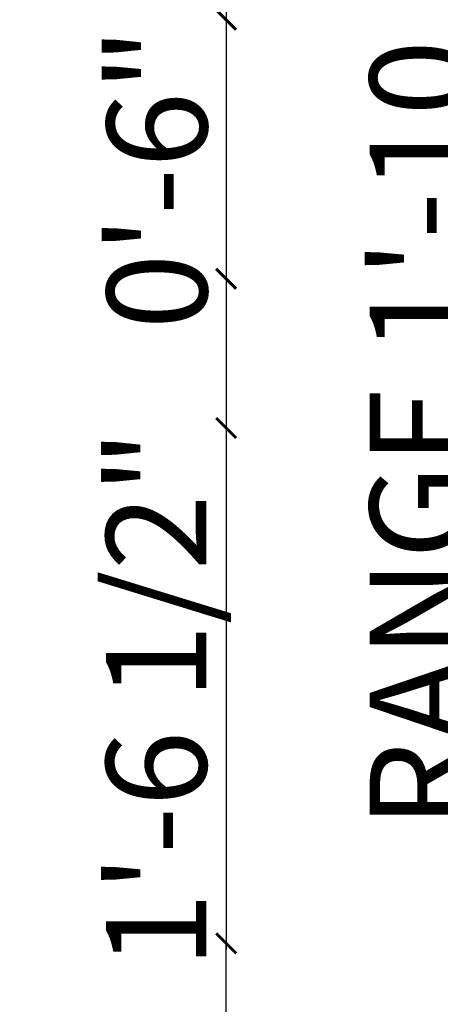
# Model space of a CAD drawing. Units: inches. Extents: x 2419 to 2878, y 1068 to 1713.
# Tile 2 of 20: x 2419 to 2471, y 1286 to 1409. Entities that reach past the tile are written whole.
import ezdxf

# ---------------------------------------------------------------- set-up
doc = ezdxf.new("R2010")
doc.units = ezdxf.units.IN
doc.layers.add('A-ANNO-DIMS', color=2, linetype='Continuous', lineweight=18)
doc.styles.get("Standard").update_dxf_attribs({"font": 'arial.ttf'})
doc.dimstyles.new('ISO-25', dxfattribs={"dimtxt": 12.5, "dimasz": 2.5, "dimexe": 1.25, "dimexo": 0.625, "dimtad": 1, "dimdec": 0, "dimlunit": 4, "dimtxsty": 'Standard', "dimblk": 'ARCHTICK', "dimcen": 2.5, "dimse1": 1, "dimse2": 1, "dimclrd": 4, "dimadec": 0, "dimazin": 0, "dimtfac": 1, "dimtdec": 0, "dimtmove": 0, "dimatfit": 3, "dimfxl": 1, "dimarcsym": 0})

# ---------------------------------------------------------------- blocks, each defined once
blk = doc.blocks.new('_ArchTick')
at = {"color": 0, "linetype": 'ByBlock', "const_width": 0.15}
blk.add_lwpolyline([(-0.5, -0.5), (0.5, 0.5)], dxfattribs=at)
blk = doc.blocks.new('*D27')
at = {"layer": 'A-ANNO-DIMS', "color": 4, "lineweight": -2, "transparency": 16777216}
for p, q in [((2493.67, 1347.69), (2493.67, 1413.78)), ((2493.67, 1311.01), (2493.67, 1347.69))]:
    blk.add_line(p, q, dxfattribs=at)
at = {"layer": 'Defpoints', "color": 0, "transparency": 16777216}
for p in [(2493.67, 1347.69), (2502.77, 1347.69), (2502.77, 1311.01)]:
    blk.add_point(p, dxfattribs=at)
at = {"layer": 'A-ANNO-DIMS', "color": 4, "lineweight": -2, "transparency": 16777216, "xscale": 2.5, "yscale": 2.5, "zscale": 2.5}
for p, rotation in [((2493.67, 1347.69), 90), ((2493.67, 1311.01), 270)]:
    blk.add_blockref('_ArchTick', p, dxfattribs=dict(at, rotation=rotation))
at = {"layer": 'A-ANNO-DIMS', "color": 0, "transparency": 16777216, "insert": (2486.57, 1381.99), "char_height": 12.5, "attachment_point": 5, "rotation": 90}
blk.add_mtext('3\'-0 1/2"', dxfattribs=at)
blk = doc.blocks.new('*D28')
at = {"layer": 'A-ANNO-DIMS', "color": 4, "lineweight": -2, "transparency": 16777216}
for p, q in [((2477.16, 1470.63), (2477.16, 1448.27)), ((2477.16, 1448.27), (2477.16, 1306.15))]:
    blk.add_line(p, q, dxfattribs=at)
at = {"layer": 'Defpoints', "color": 0, "transparency": 16777216}
for p in [(2480.51, 1470.63), (2477.16, 1448.27), (2480.51, 1448.27)]:
    blk.add_point(p, dxfattribs=at)
at = {"layer": 'A-ANNO-DIMS', "color": 4, "lineweight": -2, "transparency": 16777216, "xscale": 2.5, "yscale": 2.5, "zscale": 2.5}
for p, rotation in [((2477.16, 1470.63), 90), ((2477.16, 1448.27), 270)]:
    blk.add_blockref('_ArchTick', p, dxfattribs=dict(at, rotation=rotation))
at = {"layer": 'A-ANNO-DIMS', "color": 0, "transparency": 16777216, "insert": (2470.07, 1375.96), "char_height": 12.5, "attachment_point": 5, "rotation": 90}
blk.add_mtext('RANGE 1\'-10 1/2"', dxfattribs=at)
blk = doc.blocks.new('*D47')
at = {"layer": 'A-ANNO-DIMS', "color": 4, "lineweight": -2, "transparency": 16777216}
for p, q in [((2444.31, 1376.56), (2444.31, 1357.98)), ((2444.31, 1357.98), (2444.31, 1293.05))]:
    blk.add_line(p, q, dxfattribs=at)
at = {"layer": 'Defpoints', "color": 0, "transparency": 16777216}
for p in [(2632.51, 1376.56), (2444.31, 1357.98), (2632.51, 1357.98)]:
    blk.add_point(p, dxfattribs=at)
at = {"layer": 'A-ANNO-DIMS', "color": 4, "lineweight": -2, "transparency": 16777216, "xscale": 2.5, "yscale": 2.5, "zscale": 2.5}
for p, rotation in [((2444.31, 1376.56), 90), ((2444.31, 1357.98), 270)]:
    blk.add_blockref('_ArchTick', p, dxfattribs=dict(at, rotation=rotation))
at = {"layer": 'A-ANNO-DIMS', "color": 0, "transparency": 16777216, "insert": (2437.23, 1324.26), "char_height": 12.5, "attachment_point": 5, "rotation": 90}
blk.add_mtext('1\'-6 1/2"', dxfattribs=at)
blk = doc.blocks.new('*D54')
at = {"layer": 'A-ANNO-DIMS', "color": 4, "lineweight": -2, "transparency": 16777216}
blk.add_line((2444.31, 1130.81), (2444.31, 1293.81), dxfattribs=at)
at = {"layer": 'Defpoints', "color": 0, "transparency": 16777216}
for p in [(2444.31, 1293.81), (2480.51, 1293.81), (2480.51, 1130.81)]:
    blk.add_point(p, dxfattribs=at)
at = {"layer": 'A-ANNO-DIMS', "color": 4, "lineweight": -2, "transparency": 16777216, "xscale": 2.5, "yscale": 2.5, "zscale": 2.5}
for p, rotation in [((2444.31, 1293.81), 90), ((2444.31, 1130.81), 270)]:
    blk.add_blockref('_ArchTick', p, dxfattribs=dict(at, rotation=rotation))
at = {"layer": 'A-ANNO-DIMS', "color": 0, "transparency": 16777216, "insert": (2437.3, 1212.31), "char_height": 12.5, "attachment_point": 5, "rotation": 90}
blk.add_mtext('13\'-7"', dxfattribs=at)
blk = doc.blocks.new('*D55')
at = {"layer": 'A-ANNO-DIMS', "color": 4, "lineweight": -2, "transparency": 16777216}
for p, q in [((2444.31, 1414.81), (2444.31, 1408.81)), ((2444.31, 1408.81), (2444.31, 1371.83))]:
    blk.add_line(p, q, dxfattribs=at)
at = {"layer": 'Defpoints', "color": 0, "transparency": 16777216}
for p in [(2480.51, 1414.81), (2444.31, 1408.81), (2480.51, 1408.81)]:
    blk.add_point(p, dxfattribs=at)
at = {"layer": 'A-ANNO-DIMS', "color": 4, "lineweight": -2, "transparency": 16777216, "xscale": 2.5, "yscale": 2.5, "zscale": 2.5}
for p, rotation in [((2444.31, 1414.81), 90), ((2444.31, 1408.81), 270)]:
    blk.add_blockref('_ArchTick', p, dxfattribs=dict(at, rotation=rotation))
at = {"layer": 'A-ANNO-DIMS', "color": 0, "transparency": 16777216, "insert": (2437.31, 1389.07), "char_height": 12.5, "attachment_point": 5, "rotation": 90}
blk.add_mtext('0\'-6"', dxfattribs=at)

msp = doc.modelspace()

# ---------------------------------------------------------------- dimensions: what is measured, and where the dimension line sits
at = {"layer": 'A-ANNO-DIMS'}
dim = msp.add_linear_dim(base=(2477.16, 1448.27), p1=(2480.51, 1470.63), p2=(2480.51, 1448.27), angle=270, text='RANGE <>', dimstyle='ISO-25', override={"dimdec": 1, "dimlfac": 1, "dimrnd": 0, "dimzin": 1, "dimdsep": 46, "dimlunit": 4, "dimfrac": 2}, dxfattribs=at)
dim.commit()
dim.dimension.update_dxf_attribs({"geometry": '*D28', "text_midpoint": (2470.07, 1375.96)})
for base, p1, p2, picture, middle in [((2444.31, 1408.81), (2480.51, 1414.81), (2480.51, 1408.81), '*D55', (2437.31, 1389.07)), ((2493.67, 1347.69), (2502.77, 1311.01), (2502.77, 1347.69), '*D27', (2486.57, 1381.99)), ((2444.31, 1357.98), (2632.51, 1376.56), (2632.51, 1357.98), '*D47', (2437.23, 1324.26)), ((2444.31, 1293.81), (2480.51, 1130.81), (2480.51, 1293.81), '*D54', (2437.3, 1212.31))]:
    dim = msp.add_linear_dim(base=base, p1=p1, p2=p2, angle=90, dimstyle='ISO-25', override={"dimdec": 1, "dimlfac": 1, "dimrnd": 0, "dimzin": 1, "dimdsep": 46, "dimlunit": 4, "dimfrac": 2}, dxfattribs=at)
    dim.commit()
    dim.dimension.update_dxf_attribs({"geometry": picture, "text_midpoint": middle})

doc.saveas('drawing.dxf')
